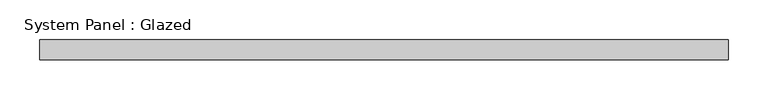
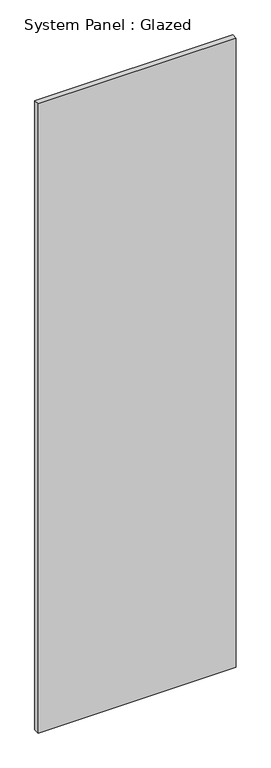
"""IFC4 building model written with IfcOpenShell, lengths in millimetres: plate geometry, System Panel : Glazed."""

from ifc_helpers import new_model, si_unit, origin, origin_with_axes, place, context, project, spatial, polyline, outline, extrude, source, transform, mapped, element, save


def system_panel_glazed_640eda3d(model_context):
    return source(origin(), model_context, "Body", "SweptSolid", [
        extrude(outline(polyline([(434.975, 19.05), (-434.975, 19.05), (-434.975, 44.45), (434.975, 44.45), (434.975, 19.05)])), origin_with_axes(), (0.0, 0.0, 1.0), 2921.0),
    ])


if __name__ == "__main__":
    model = new_model("IFC4")
    model_context = context("Model", 3, world=origin())
    ifc_project = project(units=[si_unit("LENGTHUNIT", "METRE", prefix="MILLI")], contexts=[model_context])
    site = spatial("IfcSite", under=ifc_project)
    building = spatial("IfcBuilding", under=site)
    placement = place(None, origin())
    system_panel_glazed_shape = system_panel_glazed_640eda3d(model_context)
    element("IfcPlate", 1, ObjectType="System Panel : Glazed", at=placement, inside=building, context=model_context, shape_type="MappedRepresentation", body=[
        mapped(system_panel_glazed_shape, transform((0.0, 0.0, 0.0), x_axis=(1.0, 0.0, 0.0), y_axis=(0.0, 1.0, 0.0), z_axis=(0.0, 0.0, 1.0))),
    ])
    save(model, "model.ifc")

# Revit data of these elements
# Type "System Panel : Glazed"
#   Construction Type Id = "GSP4R"
#   Analytic Construction = "1/8 in Pilkington single glazing"
#   Visual Light Transmittance = 0.9
#   Solar Heat Gain Coefficient = 0.86
#   Heat Transfer Coefficient (U) = 1.18115 BTU/(h·ft²·°F)
# Element 1 (IfcPlate, "System Panel : Glazed")
#   Materials on its faces: "Glass"
# Materials
#   "Glass": class "Glass", colour RGB 0 128 192, transparency 0.75, Description = "Soda Lime Glass", Cost = 0
